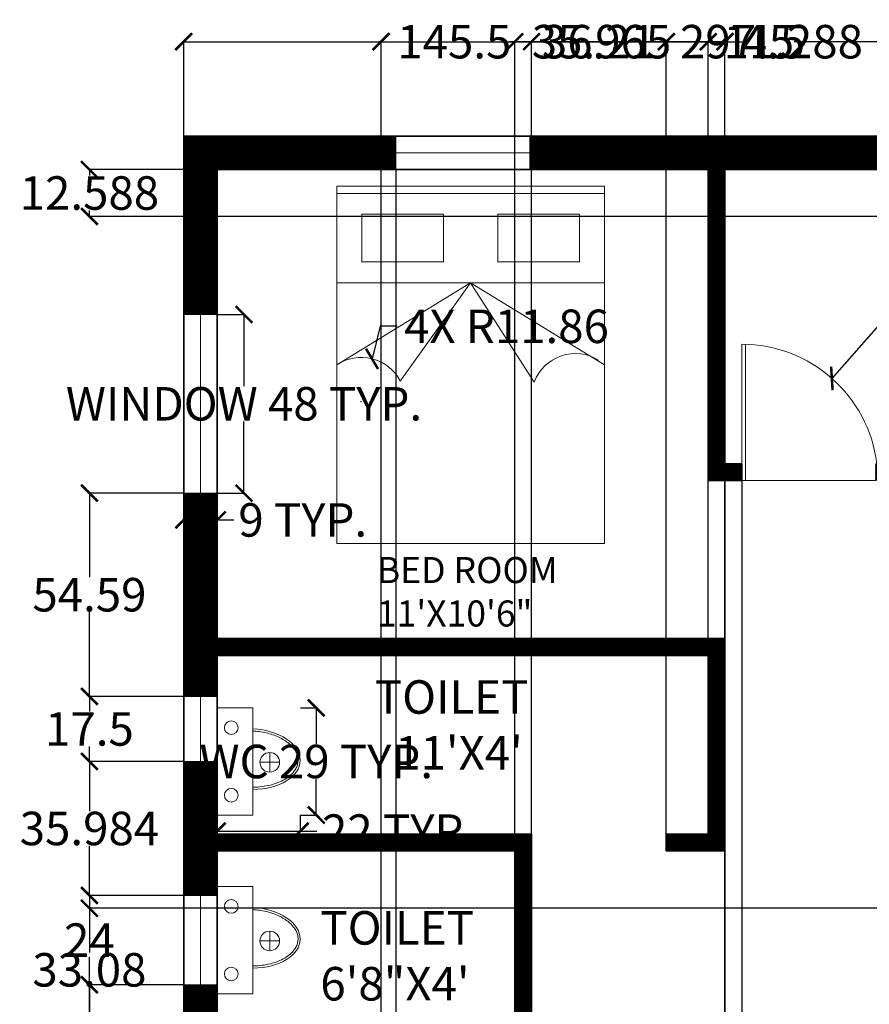
# Model space of a CAD drawing. Units: inches. Extents: x -1 to 426, y -6 to 532.
# Tile 3 of 4: x -1 to 228, y 267 to 532. Entities that reach past the tile are written whole.
import ezdxf

# ---------------------------------------------------------------- set-up
doc = ezdxf.new("R2010")
doc.units = ezdxf.units.IN
doc.header["$MEASUREMENT"] = 0
for name, color, linetype, lineweight in [('A-ANNO-DIMS', 2, 'Continuous', 18), ('A-AREA-IDEN', 7, 'Continuous', 25), ('A-DOOR', 3, 'Continuous', 18), ('A-FLOR-FIXT', 8, 'Continuous', 18), ('A-FURN', 8, 'Continuous', 18), ('A-GLAZ', 4, 'Continuous', 18)]:
    doc.layers.add(name, color=color, linetype=linetype, lineweight=lineweight)
doc.layers.add('A-WALL', color=159, linetype='Continuous', lineweight=35, true_color=0x223569)
doc.layers.add('A-WALL-PATT', color=177, linetype='Continuous', lineweight=13, true_color=0x2c4178)
doc.styles.get("Standard").update_dxf_attribs({"font": 'arial.ttf'})
doc.dimstyles.get("Standard").update_dxf_attribs({"dimtxt": 9, "dimasz": 4.5, "dimexe": 0.18, "dimexo": 0.0625, "dimgap": 0.09, "dimtad": 0, "dimtih": 1, "dimtoh": 1, "dimdec": 1, "dimzin": 0, "dimdsep": 46, "dimlunit": 4, "dimtxsty": 'Standard', "dimblk": 'ARCHTICK', "dimcen": 0.09, "dimadec": 0, "dimazin": 0, "dimtfac": 1, "dimtdec": 1, "dimtofl": 0, "dimtmove": 0, "dimatfit": 3, "dimfxl": 1, "dimtolj": 1, "dimtzin": 0, "dimarcsym": 0})

# ---------------------------------------------------------------- blocks, each defined once
blk = doc.blocks.new('WIN-36IN')
for p, q in [((0, 4.5), (36, 4.5)), ((0, -4.5), (0, 4.5)), ((36, 4.5), (36, -4.5)), ((0, 0), (36, 0)), ((36, -4.5), (0, -4.5))]:
    blk.add_line(p, q)
blk = doc.blocks.new('WIN-48IN')
for p, q in [((-4.5, 48), (4.5, 48)), ((-4.5, 0), (-4.5, 48)), ((0, 48), (0, 0)), ((4.5, 48), (4.5, 0)), ((4.5, 0), (-4.5, 0))]:
    blk.add_line(p, q)
blk = doc.blocks.new('BED-DOUBLE')
for p, q in [((-96, 0), (-96, 72)), ((-96, 72), (0, 72)), ((-26, 36), (-48, 72)), ((-26, 72), (-26, 0)), ((-2, 72), (-2, 0)), ((0, 72), (0, 0)), ((-52.33, 54.93), (-26, 36)), ((-26, 36), (-52.6, 18.9)), ((-48, 0), (-26, 36)), ((0, 0), (-96, 0))]:
    blk.add_line(p, q)
for points in [[(-7.5, 65.27), (-7.5, 43.28), (-20.33, 43.28), (-20.33, 65.27)], [(-7.5, 6.73), (-7.5, 28.72), (-20.33, 28.72), (-20.33, 6.73)]]:
    blk.add_lwpolyline(points, close=True)
for centre, start, end in [((-57.86, 65.42), 297.83, 33.7219), ((-56.81, 7.81), 328.371, 69.2037)]:
    blk.add_arc(centre, 11.86, start, end)
blk = doc.blocks.new('WC-TANK')
for p, q in [((0, -14.38), (0, 14.38)), ((0, 14.38), (9.6, 14.38)), ((9.6, 14.38), (9.6, 8.78)), ((9.6, -7.49), (9.6, 8.78)), ((14.13, -0.21), (14.13, 2.42)), ((14.13, 2.42), (14.13, -0.21)), ((14.13, -0.21), (11.49, -0.21)), ((11.49, -0.21), (14.13, -0.21)), ((14.13, -0.21), (16.76, -0.21)), ((16.76, -0.21), (14.13, -0.21)), ((14.13, -0.21), (14.13, -2.85)), ((9.6, -7.49), (9.6, -14.38)), ((9.6, -14.38), (0, -14.38))]:
    blk.add_line(p, q)
for centre, radius in [((3.77, 9.08), 1.84), ((14.13, -0.21), 2.63), ((3.77, -9.08), 1.84)]:
    blk.add_circle(centre, radius)
blk.add_ellipse((8.96, 0.66), major_axis=(13.35, -0.55), ratio=0.609473, start_param=4.785392, end_param=7.831087)
blk.add_open_spline([(9.6, -6.9), (10.03, -6.9), (10.47, -6.89), (11.69, -6.81), (12.46, -6.71), (13.95, -6.44), (14.67, -6.26), (16.04, -5.82), (16.69, -5.56), (17.88, -4.98), (18.43, -4.66), (19.41, -3.96), (19.84, -3.58), (20.51, -2.87), (20.76, -2.54), (21.18, -1.86), (21.35, -1.52), (21.59, -0.82), (21.67, -0.47), (21.74, 0.24), (21.73, 0.6), (21.63, 1.32), (21.53, 1.67), (21.25, 2.39), (21.07, 2.74), (20.61, 3.44), (20.33, 3.79), (19.7, 4.45), (19.34, 4.77), (18.55, 5.39), (18.12, 5.68), (17.18, 6.22), (16.67, 6.48), (15.61, 6.94), (15.05, 7.14), (13.89, 7.51), (13.29, 7.66), (12.06, 7.92), (11.43, 8.02), (10.38, 8.14), (9.98, 8.18), (9.57, 8.2)], degree=3, knots=[4.785392, 4.785392, 4.785392, 4.785392, 4.886226, 4.886226, 5.069344, 5.069344, 5.252462, 5.252462, 5.43558, 5.43558, 5.618699, 5.618699, 5.801817, 5.801817, 5.950651, 5.950651, 6.099486, 6.099486, 6.248321, 6.248321, 6.397155, 6.397155, 6.54599, 6.54599, 6.694824, 6.694824, 6.843659, 6.843659, 6.992494, 6.992494, 7.141328, 7.141328, 7.290163, 7.290163, 7.438998, 7.438998, 7.587832, 7.587832, 7.736667, 7.736667, 7.831087, 7.831087, 7.831087, 7.831087])
blk = doc.blocks.new('_ArchTick')
at = {"color": 0, "linetype": 'ByBlock', "const_width": 0.15}
blk.add_lwpolyline([(-0.5, -0.5), (0.5, 0.5)], dxfattribs=at)
blk = doc.blocks.new('*D9')
at = {"layer": 'A-ANNO-DIMS', "color": 0, "lineweight": -2, "transparency": 16777216}
for p, q in [((52.39, 452.57), (59.7, 452.57)), ((59.52, 452.57), (59.52, 433.32)), ((59.52, 404.57), (59.52, 423.82)), ((52.39, 404.57), (59.7, 404.57))]:
    blk.add_line(p, q, dxfattribs=at)
at = {"layer": 'Defpoints', "color": 0, "transparency": 16777216}
for p in [(52.32, 452.57), (59.52, 452.57), (52.32, 404.57)]:
    blk.add_point(p, dxfattribs=at)
at = {"layer": 'A-ANNO-DIMS', "color": 0, "lineweight": -2, "transparency": 16777216, "xscale": 4.5, "yscale": 4.5, "zscale": 4.5}
for p, rotation in [((59.52, 452.57), 90), ((59.52, 404.57), 270)]:
    blk.add_blockref('_ArchTick', p, dxfattribs=dict(at, rotation=rotation))
at = {"layer": 'A-ANNO-DIMS', "color": 0, "transparency": 16777216, "insert": (59.52, 428.57), "char_height": 9, "attachment_point": 5}
blk.add_mtext('\\A1;WINDOW 48 TYP.', dxfattribs=at)
blk = doc.blocks.new('*D10')
at = {"layer": 'A-ANNO-DIMS', "color": 0, "lineweight": -2, "transparency": 16777216}
for p, q in [((43.32, 404.51), (43.32, 397.19)), ((52.32, 404.51), (52.32, 397.19)), ((43.32, 397.37), (52.32, 397.37)), ((52.32, 397.37), (56.82, 397.37))]:
    blk.add_line(p, q, dxfattribs=at)
at = {"layer": 'Defpoints', "color": 0, "transparency": 16777216}
for p in [(43.32, 404.57), (52.32, 404.57), (52.32, 397.37)]:
    blk.add_point(p, dxfattribs=at)
at = {"layer": 'A-ANNO-DIMS', "color": 0, "lineweight": -2, "transparency": 16777216, "xscale": 4.5, "yscale": 4.5, "zscale": 4.5, "rotation": 180}
blk.add_blockref('_ArchTick', (43.32, 397.37), dxfattribs=at)
at = {"layer": 'A-ANNO-DIMS', "color": 0, "lineweight": -2, "transparency": 16777216, "xscale": 4.5, "yscale": 4.5, "zscale": 4.5}
blk.add_blockref('_ArchTick', (52.32, 397.37), dxfattribs=at)
at = {"layer": 'A-ANNO-DIMS', "color": 0, "transparency": 16777216, "insert": (75.32, 397.37), "char_height": 9, "attachment_point": 5}
blk.add_mtext('\\A1;9 TYP.', dxfattribs=at)
blk = doc.blocks.new('*D13')
at = {"layer": 'A-ANNO-DIMS', "color": 0, "lineweight": -2, "transparency": 16777216}
for p, q in [((74.7, 346.87), (79.13, 346.87)), ((78.95, 346.87), (78.95, 337.23)), ((78.95, 318.1), (78.95, 327.74)), ((74.7, 318.1), (79.13, 318.1))]:
    blk.add_line(p, q, dxfattribs=at)
at = {"layer": 'Defpoints', "color": 0, "transparency": 16777216}
for p in [(74.64, 346.87), (78.95, 346.87), (74.64, 318.1)]:
    blk.add_point(p, dxfattribs=at)
at = {"layer": 'A-ANNO-DIMS', "color": 0, "lineweight": -2, "transparency": 16777216, "xscale": 4.5, "yscale": 4.5, "zscale": 4.5}
for p, rotation in [((78.95, 346.87), 90), ((78.95, 318.1), 270)]:
    blk.add_blockref('_ArchTick', p, dxfattribs=dict(at, rotation=rotation))
at = {"layer": 'A-ANNO-DIMS', "color": 0, "transparency": 16777216, "insert": (78.95, 332.48), "char_height": 9, "attachment_point": 5}
blk.add_mtext('\\A1;WC 29 TYP.', dxfattribs=at)
blk = doc.blocks.new('*D14')
at = {"layer": 'A-ANNO-DIMS', "color": 0, "lineweight": -2, "transparency": 16777216}
for p, q in [((52.32, 318.03), (52.32, 313.6)), ((74.64, 318.03), (74.64, 313.6)), ((52.32, 313.78), (74.64, 313.78)), ((74.64, 313.78), (79.14, 313.78))]:
    blk.add_line(p, q, dxfattribs=at)
at = {"layer": 'Defpoints', "color": 0, "transparency": 16777216}
for p in [(52.32, 318.1), (74.64, 318.1), (74.64, 313.78)]:
    blk.add_point(p, dxfattribs=at)
at = {"layer": 'A-ANNO-DIMS', "color": 0, "lineweight": -2, "transparency": 16777216, "xscale": 4.5, "yscale": 4.5, "zscale": 4.5, "rotation": 180}
blk.add_blockref('_ArchTick', (52.32, 313.78), dxfattribs=at)
at = {"layer": 'A-ANNO-DIMS', "color": 0, "lineweight": -2, "transparency": 16777216, "xscale": 4.5, "yscale": 4.5, "zscale": 4.5}
blk.add_blockref('_ArchTick', (74.64, 313.78), dxfattribs=at)
at = {"layer": 'A-ANNO-DIMS', "color": 0, "transparency": 16777216, "insert": (101.21, 313.78), "char_height": 9, "attachment_point": 5}
blk.add_mtext('\\A1;22 TYP.', dxfattribs=at)
blk = doc.blocks.new('*D17')
at = {"layer": 'A-ANNO-DIMS', "color": 0, "lineweight": -2, "transparency": 16777216}
for p, q in [((43.32, 500.54), (43.32, 526.02)), ((43.32, 525.84), (176.69, 525.84)), ((340.82, 525.84), (207.46, 525.84)), ((340.82, 500.54), (340.82, 526.02))]:
    blk.add_line(p, q, dxfattribs=at)
at = {"layer": 'Defpoints', "color": 0, "transparency": 16777216}
for p in [(340.82, 525.84), (43.32, 500.48), (340.82, 500.48)]:
    blk.add_point(p, dxfattribs=at)
at = {"layer": 'A-ANNO-DIMS', "color": 0, "lineweight": -2, "transparency": 16777216, "xscale": 4.5, "yscale": 4.5, "zscale": 4.5, "rotation": 180}
blk.add_blockref('_ArchTick', (43.32, 525.84), dxfattribs=at)
at = {"layer": 'A-ANNO-DIMS', "color": 0, "lineweight": -2, "transparency": 16777216, "xscale": 4.5, "yscale": 4.5, "zscale": 4.5}
blk.add_blockref('_ArchTick', (340.82, 525.84), dxfattribs=at)
at = {"layer": 'A-ANNO-DIMS', "color": 0, "transparency": 16777216, "insert": (192.07, 525.84), "char_height": 9, "attachment_point": 5}
blk.add_mtext('\\A1;297.5', dxfattribs=at)
blk = doc.blocks.new('*D20')
at = {"layer": 'A-ANNO-DIMS', "color": 0, "lineweight": -2, "transparency": 16777216}
for p, q in [((43.32, 67.04), (43.32, 526.02)), ((43.32, 525.84), (101.19, 525.84)), ((188.82, 525.84), (130.96, 525.84)), ((188.82, 67.04), (188.82, 526.02))]:
    blk.add_line(p, q, dxfattribs=at)
at = {"layer": 'Defpoints', "color": 0, "transparency": 16777216}
for p in [(188.82, 525.84), (43.32, 66.98), (188.82, 66.98)]:
    blk.add_point(p, dxfattribs=at)
at = {"layer": 'A-ANNO-DIMS', "color": 0, "lineweight": -2, "transparency": 16777216, "xscale": 4.5, "yscale": 4.5, "zscale": 4.5, "rotation": 180}
blk.add_blockref('_ArchTick', (43.32, 525.84), dxfattribs=at)
at = {"layer": 'A-ANNO-DIMS', "color": 0, "lineweight": -2, "transparency": 16777216, "xscale": 4.5, "yscale": 4.5, "zscale": 4.5}
blk.add_blockref('_ArchTick', (188.82, 525.84), dxfattribs=at)
at = {"layer": 'A-ANNO-DIMS', "color": 0, "transparency": 16777216, "insert": (116.07, 525.84), "char_height": 9, "attachment_point": 5}
blk.add_mtext('\\A1;145.5', dxfattribs=at)
blk = doc.blocks.new('*D22')
at = {"layer": 'A-ANNO-DIMS', "color": 0, "lineweight": -2, "transparency": 16777216}
for p, q in [((52.32, 491.42), (52.32, 5.45)), ((100.32, 491.42), (100.32, 5.45)), ((52.32, 5.63), (69.6, 5.63)), ((100.32, 5.63), (83.05, 5.63))]:
    blk.add_line(p, q, dxfattribs=at)
at = {"layer": 'Defpoints', "color": 0, "transparency": 16777216}
for p in [(52.32, 491.48), (100.32, 491.48), (100.32, 5.63)]:
    blk.add_point(p, dxfattribs=at)
at = {"layer": 'A-ANNO-DIMS', "color": 0, "lineweight": -2, "transparency": 16777216, "xscale": 4.5, "yscale": 4.5, "zscale": 4.5, "rotation": 180}
blk.add_blockref('_ArchTick', (52.32, 5.63), dxfattribs=at)
at = {"layer": 'A-ANNO-DIMS', "color": 0, "lineweight": -2, "transparency": 16777216, "xscale": 4.5, "yscale": 4.5, "zscale": 4.5}
blk.add_blockref('_ArchTick', (100.32, 5.63), dxfattribs=at)
at = {"layer": 'A-ANNO-DIMS', "color": 0, "transparency": 16777216, "insert": (76.32, 5.63), "char_height": 9, "attachment_point": 5}
blk.add_mtext('\\A1;48', dxfattribs=at)
blk = doc.blocks.new('*D26')
at = {"layer": 'A-ANNO-DIMS', "color": 0, "lineweight": -2, "transparency": 16777216}
for p, q in [((43.26, 272.5), (17.79, 272.5)), ((17.97, 272.5), (17.97, 234.11)), ((17.97, 186.36), (17.97, 224.74)), ((43.26, 186.36), (17.79, 186.36))]:
    blk.add_line(p, q, dxfattribs=at)
at = {"layer": 'Defpoints', "color": 0, "transparency": 16777216}
for p in [(17.97, 272.5), (43.32, 272.5), (43.32, 186.36)]:
    blk.add_point(p, dxfattribs=at)
at = {"layer": 'A-ANNO-DIMS', "color": 0, "lineweight": -2, "transparency": 16777216, "xscale": 4.5, "yscale": 4.5, "zscale": 4.5}
for p, rotation in [((17.97, 272.5), 90), ((17.97, 186.36), 270)]:
    blk.add_blockref('_ArchTick', p, dxfattribs=dict(at, rotation=rotation))
at = {"layer": 'A-ANNO-DIMS', "color": 0, "transparency": 16777216, "insert": (17.97, 229.43), "char_height": 9, "attachment_point": 5}
blk.add_mtext('\\A1;86.14', dxfattribs=at)
blk = doc.blocks.new('*D27')
at = {"layer": 'A-ANNO-DIMS', "color": 0, "lineweight": -2, "transparency": 16777216}
for p, q in [((43.26, 296.5), (17.79, 296.5)), ((17.97, 296.5), (17.97, 289.11)), ((17.97, 272.5), (17.97, 279.89)), ((43.26, 272.5), (17.79, 272.5))]:
    blk.add_line(p, q, dxfattribs=at)
at = {"layer": 'Defpoints', "color": 0, "transparency": 16777216}
for p in [(17.97, 296.5), (43.32, 296.5), (43.32, 272.5)]:
    blk.add_point(p, dxfattribs=at)
at = {"layer": 'A-ANNO-DIMS', "color": 0, "lineweight": -2, "transparency": 16777216, "xscale": 4.5, "yscale": 4.5, "zscale": 4.5}
for p, rotation in [((17.97, 296.5), 90), ((17.97, 272.5), 270)]:
    blk.add_blockref('_ArchTick', p, dxfattribs=dict(at, rotation=rotation))
at = {"layer": 'A-ANNO-DIMS', "color": 0, "transparency": 16777216, "insert": (17.97, 284.5), "char_height": 9, "attachment_point": 5}
blk.add_mtext('\\A1;24', dxfattribs=at)
blk = doc.blocks.new('*D28')
at = {"layer": 'A-ANNO-DIMS', "color": 0, "lineweight": -2, "transparency": 16777216}
for p, q in [((43.26, 332.48), (17.79, 332.48)), ((17.97, 332.48), (17.97, 319.18)), ((17.97, 296.5), (17.97, 309.8)), ((43.26, 296.5), (17.79, 296.5))]:
    blk.add_line(p, q, dxfattribs=at)
at = {"layer": 'Defpoints', "color": 0, "transparency": 16777216}
for p in [(17.97, 332.48), (43.32, 332.48), (43.32, 296.5)]:
    blk.add_point(p, dxfattribs=at)
at = {"layer": 'A-ANNO-DIMS', "color": 0, "lineweight": -2, "transparency": 16777216, "xscale": 4.5, "yscale": 4.5, "zscale": 4.5}
for p, rotation in [((17.97, 332.48), 90), ((17.97, 296.5), 270)]:
    blk.add_blockref('_ArchTick', p, dxfattribs=dict(at, rotation=rotation))
at = {"layer": 'A-ANNO-DIMS', "color": 0, "transparency": 16777216, "insert": (17.97, 314.49), "char_height": 9, "attachment_point": 5}
blk.add_mtext('\\A1;35.984', dxfattribs=at)
blk = doc.blocks.new('*D29')
at = {"layer": 'A-ANNO-DIMS', "color": 0, "lineweight": -2, "transparency": 16777216}
for p, q in [((43.26, 349.98), (17.79, 349.98)), ((17.97, 349.98), (17.97, 345.92)), ((17.97, 332.48), (17.97, 336.55)), ((43.26, 332.48), (17.79, 332.48))]:
    blk.add_line(p, q, dxfattribs=at)
at = {"layer": 'Defpoints', "color": 0, "transparency": 16777216}
for p in [(17.97, 349.98), (43.32, 349.98), (43.32, 332.48)]:
    blk.add_point(p, dxfattribs=at)
at = {"layer": 'A-ANNO-DIMS', "color": 0, "lineweight": -2, "transparency": 16777216, "xscale": 4.5, "yscale": 4.5, "zscale": 4.5}
for p, rotation in [((17.97, 349.98), 90), ((17.97, 332.48), 270)]:
    blk.add_blockref('_ArchTick', p, dxfattribs=dict(at, rotation=rotation))
at = {"layer": 'A-ANNO-DIMS', "color": 0, "transparency": 16777216, "insert": (17.97, 341.23), "char_height": 9, "attachment_point": 5}
blk.add_mtext('\\A1;17.5', dxfattribs=at)
blk = doc.blocks.new('*D30')
at = {"layer": 'A-ANNO-DIMS', "color": 0, "lineweight": -2, "transparency": 16777216}
for p, q in [((43.26, 404.57), (17.79, 404.57)), ((17.97, 404.57), (17.97, 381.96)), ((17.97, 349.98), (17.97, 372.59)), ((43.26, 349.98), (17.79, 349.98))]:
    blk.add_line(p, q, dxfattribs=at)
at = {"layer": 'Defpoints', "color": 0, "transparency": 16777216}
for p in [(17.97, 404.57), (43.32, 404.57), (43.32, 349.98)]:
    blk.add_point(p, dxfattribs=at)
at = {"layer": 'A-ANNO-DIMS', "color": 0, "lineweight": -2, "transparency": 16777216, "xscale": 4.5, "yscale": 4.5, "zscale": 4.5}
for p, rotation in [((17.97, 404.57), 90), ((17.97, 349.98), 270)]:
    blk.add_blockref('_ArchTick', p, dxfattribs=dict(at, rotation=rotation))
at = {"layer": 'A-ANNO-DIMS', "color": 0, "transparency": 16777216, "insert": (17.97, 377.28), "char_height": 9, "attachment_point": 5}
blk.add_mtext('\\A1;54.59', dxfattribs=at)
blk = doc.blocks.new('*D32')
at = {"layer": 'A-ANNO-DIMS', "color": 0, "lineweight": -2, "transparency": 16777216}
for p, q in [((331.76, 293.06), (17.79, 293.06)), ((17.97, 293.06), (17.97, 281.21)), ((17.97, 259.98), (17.97, 271.83)), ((331.76, 259.98), (17.79, 259.98))]:
    blk.add_line(p, q, dxfattribs=at)
at = {"layer": 'Defpoints', "color": 0, "transparency": 16777216}
for p in [(17.97, 293.06), (331.82, 293.06), (331.82, 259.98)]:
    blk.add_point(p, dxfattribs=at)
at = {"layer": 'A-ANNO-DIMS', "color": 0, "lineweight": -2, "transparency": 16777216, "xscale": 4.5, "yscale": 4.5, "zscale": 4.5}
for p, rotation in [((17.97, 293.06), 90), ((17.97, 259.98), 270)]:
    blk.add_blockref('_ArchTick', p, dxfattribs=dict(at, rotation=rotation))
at = {"layer": 'A-ANNO-DIMS', "color": 0, "transparency": 16777216, "insert": (17.97, 276.52), "char_height": 9, "attachment_point": 5}
blk.add_mtext('\\A1;33.08', dxfattribs=at)
blk = doc.blocks.new('*D33')
at = {"layer": 'A-ANNO-DIMS', "color": 0, "lineweight": -2, "transparency": 16777216}
for p, q in [((331.76, 491.48), (17.79, 491.48)), ((17.97, 491.48), (17.97, 489.87)), ((331.76, 478.89), (17.79, 478.89)), ((17.97, 478.89), (17.97, 480.5))]:
    blk.add_line(p, q, dxfattribs=at)
at = {"layer": 'Defpoints', "color": 0, "transparency": 16777216}
for p in [(17.97, 491.48), (331.82, 491.48), (331.82, 478.89)]:
    blk.add_point(p, dxfattribs=at)
at = {"layer": 'A-ANNO-DIMS', "color": 0, "lineweight": -2, "transparency": 16777216, "xscale": 4.5, "yscale": 4.5, "zscale": 4.5}
for p, rotation in [((17.97, 491.48), 90), ((17.97, 478.89), 270)]:
    blk.add_blockref('_ArchTick', p, dxfattribs=dict(at, rotation=rotation))
at = {"layer": 'A-ANNO-DIMS', "color": 0, "transparency": 16777216, "insert": (17.97, 485.19), "char_height": 9, "attachment_point": 5}
blk.add_mtext('\\A1;12.588', dxfattribs=at)
blk = doc.blocks.new('*D39')
at = {"layer": 'A-ANNO-DIMS', "color": 0, "lineweight": -2, "transparency": 16777216}
for p, q in [((96.36, 256.04), (96.36, 526.02)), ((96.36, 525.84), (132.32, 525.84)), ((132.32, 256.04), (132.32, 526.02)), ((132.32, 525.84), (136.82, 525.84))]:
    blk.add_line(p, q, dxfattribs=at)
at = {"layer": 'Defpoints', "color": 0, "transparency": 16777216}
for p in [(132.32, 525.84), (96.36, 255.98), (132.32, 255.98)]:
    blk.add_point(p, dxfattribs=at)
at = {"layer": 'A-ANNO-DIMS', "color": 0, "lineweight": -2, "transparency": 16777216, "xscale": 4.5, "yscale": 4.5, "zscale": 4.5, "rotation": 180}
blk.add_blockref('_ArchTick', (96.36, 525.84), dxfattribs=at)
at = {"layer": 'A-ANNO-DIMS', "color": 0, "lineweight": -2, "transparency": 16777216, "xscale": 4.5, "yscale": 4.5, "zscale": 4.5}
blk.add_blockref('_ArchTick', (132.32, 525.84), dxfattribs=at)
at = {"layer": 'A-ANNO-DIMS', "color": 0, "transparency": 16777216, "insert": (155.63, 525.84), "char_height": 9, "attachment_point": 5}
blk.add_mtext('\\A1;35.965', dxfattribs=at)
blk = doc.blocks.new('*D40')
at = {"layer": 'A-ANNO-DIMS', "color": 0, "lineweight": -2, "transparency": 16777216}
for p, q in [((136.82, 313.04), (136.82, 526.02)), ((136.82, 525.84), (140.53, 525.84)), ((173.04, 525.84), (169.33, 525.84)), ((173.04, 313.04), (173.04, 526.02))]:
    blk.add_line(p, q, dxfattribs=at)
at = {"layer": 'Defpoints', "color": 0, "transparency": 16777216}
for p in [(173.04, 525.84), (136.82, 312.98), (173.04, 312.98)]:
    blk.add_point(p, dxfattribs=at)
at = {"layer": 'A-ANNO-DIMS', "color": 0, "lineweight": -2, "transparency": 16777216, "xscale": 4.5, "yscale": 4.5, "zscale": 4.5, "rotation": 180}
blk.add_blockref('_ArchTick', (136.82, 525.84), dxfattribs=at)
at = {"layer": 'A-ANNO-DIMS', "color": 0, "lineweight": -2, "transparency": 16777216, "xscale": 4.5, "yscale": 4.5, "zscale": 4.5}
blk.add_blockref('_ArchTick', (173.04, 525.84), dxfattribs=at)
at = {"layer": 'A-ANNO-DIMS', "color": 0, "transparency": 16777216, "insert": (154.93, 525.84), "char_height": 9, "attachment_point": 5}
blk.add_mtext('\\A1;36.21', dxfattribs=at)
blk = doc.blocks.new('*D41')
at = {"layer": 'A-ANNO-DIMS', "color": 0, "lineweight": -2, "transparency": 16777216}
for p, q in [((184.32, 361.04), (184.32, 526.02)), ((184.32, 525.84), (188.82, 525.84)), ((188.82, 365.54), (188.82, 526.02)), ((188.82, 525.84), (193.32, 525.84))]:
    blk.add_line(p, q, dxfattribs=at)
at = {"layer": 'Defpoints', "color": 0, "transparency": 16777216}
for p in [(188.82, 525.84), (188.82, 365.48), (184.32, 360.98)]:
    blk.add_point(p, dxfattribs=at)
at = {"layer": 'A-ANNO-DIMS', "color": 0, "lineweight": -2, "transparency": 16777216, "xscale": 4.5, "yscale": 4.5, "zscale": 4.5, "rotation": 180}
blk.add_blockref('_ArchTick', (184.32, 525.84), dxfattribs=at)
at = {"layer": 'A-ANNO-DIMS', "color": 0, "lineweight": -2, "transparency": 16777216, "xscale": 4.5, "yscale": 4.5, "zscale": 4.5}
blk.add_blockref('_ArchTick', (188.82, 525.84), dxfattribs=at)
at = {"layer": 'A-ANNO-DIMS', "color": 0, "transparency": 16777216, "insert": (201.82, 525.84), "char_height": 9, "attachment_point": 5}
blk.add_mtext('\\A1;4.5', dxfattribs=at)
blk = doc.blocks.new('*D47')
at = {"layer": 'A-ANNO-DIMS', "color": 0, "lineweight": -2, "transparency": 16777216}
for p, q in [((188.82, 412.42), (188.82, 5.45)), ((193.32, 412.42), (193.32, 5.45)), ((188.82, 5.63), (193.32, 5.63)), ((193.32, 5.63), (197.82, 5.63))]:
    blk.add_line(p, q, dxfattribs=at)
at = {"layer": 'Defpoints', "color": 0, "transparency": 16777216}
for p in [(188.82, 412.48), (193.32, 412.48), (193.32, 5.63)]:
    blk.add_point(p, dxfattribs=at)
at = {"layer": 'A-ANNO-DIMS', "color": 0, "lineweight": -2, "transparency": 16777216, "xscale": 4.5, "yscale": 4.5, "zscale": 4.5, "rotation": 180}
blk.add_blockref('_ArchTick', (188.82, 5.63), dxfattribs=at)
at = {"layer": 'A-ANNO-DIMS', "color": 0, "lineweight": -2, "transparency": 16777216, "xscale": 4.5, "yscale": 4.5, "zscale": 4.5}
blk.add_blockref('_ArchTick', (193.32, 5.63), dxfattribs=at)
at = {"layer": 'A-ANNO-DIMS', "color": 0, "transparency": 16777216, "insert": (206.32, 5.63), "char_height": 9, "attachment_point": 5}
blk.add_mtext('\\A1;4.5', dxfattribs=at)
blk = doc.blocks.new('*D50')
at = {"layer": 'A-ANNO-DIMS', "color": 0, "lineweight": -2, "transparency": 16777216}
for p, q in [((173.04, 313.04), (173.04, 526.02)), ((173.04, 525.84), (184.32, 525.84)), ((184.32, 313.04), (184.32, 526.02)), ((184.32, 525.84), (188.82, 525.84))]:
    blk.add_line(p, q, dxfattribs=at)
at = {"layer": 'Defpoints', "color": 0, "transparency": 16777216}
for p in [(184.32, 525.84), (173.04, 312.98), (184.32, 312.98)]:
    blk.add_point(p, dxfattribs=at)
at = {"layer": 'A-ANNO-DIMS', "color": 0, "lineweight": -2, "transparency": 16777216, "xscale": 4.5, "yscale": 4.5, "zscale": 4.5, "rotation": 180}
blk.add_blockref('_ArchTick', (173.04, 525.84), dxfattribs=at)
at = {"layer": 'A-ANNO-DIMS', "color": 0, "lineweight": -2, "transparency": 16777216, "xscale": 4.5, "yscale": 4.5, "zscale": 4.5}
blk.add_blockref('_ArchTick', (184.32, 525.84), dxfattribs=at)
at = {"layer": 'A-ANNO-DIMS', "color": 0, "transparency": 16777216, "insert": (207.18, 525.84), "char_height": 9, "attachment_point": 5}
blk.add_mtext('\\A1;11.288', dxfattribs=at)
blk = doc.blocks.new('*D55')
at = {"layer": 'A-ANNO-DIMS', "color": 0, "lineweight": -2, "transparency": 16777216}
for p, q in [((232.09, 451.85), (217.55, 435.4)), ((236.59, 451.85), (232.09, 451.85)), ((193.23, 407.98), (193.41, 407.98)), ((193.32, 407.89), (193.32, 408.07))]:
    blk.add_line(p, q, dxfattribs=at)
at = {"layer": 'Defpoints', "color": 0, "transparency": 16777216}
for p in [(217.55, 435.4), (193.32, 407.98)]:
    blk.add_point(p, dxfattribs=at)
at = {"layer": 'A-ANNO-DIMS', "color": 0, "lineweight": -2, "transparency": 16777216, "xscale": 4.5, "yscale": 4.5, "zscale": 4.5, "rotation": 228.5330341154112}
blk.add_blockref('_ArchTick', (217.55, 435.4), dxfattribs=at)
at = {"layer": 'A-ANNO-DIMS', "color": 0, "transparency": 16777216, "insert": (259.7, 451.85), "char_height": 9, "attachment_point": 5}
blk.add_mtext('\\A1;R36.585', dxfattribs=at)
blk = doc.blocks.new('*D57')
at = {"layer": 'A-ANNO-DIMS', "color": 0, "lineweight": -2, "transparency": 16777216}
for p, q in [((96.16, 449.38), (93.94, 440.65)), ((100.66, 449.38), (96.16, 449.38)), ((90.94, 429.15), (91.12, 429.15)), ((91.03, 429.06), (91.03, 429.24))]:
    blk.add_line(p, q, dxfattribs=at)
at = {"layer": 'Defpoints', "color": 0, "transparency": 16777216}
for p in [(93.94, 440.65), (91.03, 429.15)]:
    blk.add_point(p, dxfattribs=at)
at = {"layer": 'A-ANNO-DIMS', "color": 0, "lineweight": -2, "transparency": 16777216, "xscale": 4.5, "yscale": 4.5, "zscale": 4.5, "rotation": 255.7751302601228}
blk.add_blockref('_ArchTick', (93.94, 440.65), dxfattribs=at)
at = {"layer": 'A-ANNO-DIMS', "color": 0, "transparency": 16777216, "insert": (130.09, 449.38), "char_height": 9, "attachment_point": 5}
blk.add_mtext('\\A1;4X R11.86', dxfattribs=at)

msp = doc.modelspace()

# ---------------------------------------------------------------- hatches: boundary and pattern name
at = {"layer": 'A-WALL-PATT'}
h = msp.add_hatch(dxfattribs=at)
h.set_pattern_fill('ANSI31', color=256)
h.set_pattern_definition([(45, (-574.8435, 0), (-0.088388348, 0.088388348), [])])
h.paths.add_polyline_path([(100.3238, 500.4824), (43.3238, 500.4824), (43.3238, 452.5693), (52.3238, 452.5693), (52.3238, 491.4824), (100.3238, 491.4824)])
h.paths.add_polyline_path([(242.3238, 500.4824), (136.3238, 500.4824), (136.3238, 491.4824), (184.3238, 491.4824), (184.3238, 407.9824), (188.8238, 407.9824), (193.3238, 407.9824), (193.3238, 412.4824), (188.8238, 412.4824), (188.8238, 491.4824), (242.3238, 491.4824)])
h.paths.add_polyline_path([(340.8238, 500.4824), (278.3238, 500.4824), (278.3238, 491.4824), (331.8238, 491.4824), (331.8238, 478.8941), (340.8238, 478.8941)])
h.paths.add_polyline_path([(331.8238, 412.4824), (229.3238, 412.4824), (229.3238, 407.9824), (331.8238, 407.9824)])
h.paths.add_polyline_path([(340.8238, 430.8941), (331.8238, 430.8941), (331.8238, 341.0593), (340.8238, 341.0593)])
h.paths.add_polyline_path([(340.8238, 293.0593), (331.8238, 293.0593), (331.8238, 259.9824), (282.3238, 259.9824), (282.3238, 255.4824), (331.8238, 255.4824), (331.8238, 237.2917), (340.8238, 237.2917)])
h.paths.add_polyline_path([(340.8238, 153.5275), (340.8238, 201.2917), (331.8238, 201.2917), (331.8238, 177.4824), (241.8238, 177.4824), (241.8238, 255.4824), (246.3238, 255.4824), (246.3238, 259.9824), (237.3238, 259.9824), (237.3238, 255.4824), (237.3238, 172.9824), (331.8238, 172.9824), (331.8238, 153.5275), (331.8238, 75.9824), (237.3238, 75.9824), (237.3238, 66.9824), (340.8238, 66.9824)])
h.paths.add_polyline_path([(98.5766, 75.9824), (52.3238, 75.9824), (52.3238, 138.3606), (43.3238, 138.3606), (43.3238, 66.9824), (52.3238, 66.9824), (98.5766, 66.9824)])
h.paths.add_polyline_path([(188.8238, 75.9824), (188.8238, 153.5275), (188.8238, 209.4042, -0.02664097), (184.3238, 209.1642), (184.3238, 153.5275), (184.3238, 75.9824), (136.8238, 75.9824), (134.5766, 75.9824), (134.5766, 66.9824), (136.8238, 66.9824), (188.8238, 66.9824)])
h.paths.add_polyline_path([(52.3238, 255.9824), (96.3583, 255.9824), (96.3583, 260.4824), (52.3238, 260.4824), (52.3238, 272.4986), (43.3238, 272.4986), (43.3238, 186.3606), (52.3238, 186.3606)])
h.paths.add_polyline_path([(52.3238, 404.5693), (43.3238, 404.5693), (43.3238, 349.9808), (52.3238, 349.9808), (52.3238, 360.9824), (184.3238, 360.9824), (184.3238, 312.9824), (173.036, 312.9824), (173.036, 308.4824), (184.3238, 308.4824), (188.8238, 308.4824), (188.8238, 365.4824), (184.3238, 365.4824), (52.3238, 365.4824)])
h.paths.add_polyline_path([(188.8238, 260.4824), (136.8238, 260.4824), (136.8238, 308.4824), (136.8238, 312.9824), (52.3238, 312.9824), (52.3238, 332.4824), (43.3238, 332.4824), (43.3238, 308.4824), (43.3238, 296.4986), (52.3238, 296.4986), (52.3238, 298.8674), (52.3238, 308.4824), (132.3238, 308.4824), (132.3238, 260.4824), (132.3238, 255.9824), (136.8238, 255.9824), (184.3238, 255.9824), (184.3238, 251.4824), (186.5738, 251.4824), (188.8238, 251.4824), (188.8238, 255.9824)])

# ---------------------------------------------------------------- linework, layer by layer
at = {"layer": 'A-DOOR'}
for p, q in [((193.3238, 407.9824), (193.3238, 444.5678)), ((194.3238, 407.9824), (194.3238, 444.5541)), ((193.3238, 407.9824), (229.3238, 407.9824))]:
    msp.add_line(p, q, dxfattribs=at)
msp.add_arc((193.3238, 407.9824), 36.5854, 7.065274, 90, dxfattribs=at)
at = {"layer": 'A-GLAZ'}
for p, q in [((43.3238, 349.9808), (52.3238, 349.9808)), ((43.3238, 325.9808), (43.3238, 349.9808)), ((47.8238, 349.9808), (47.8238, 332.4824)), ((52.3238, 349.9808), (52.3238, 325.9808)), ((43.3238, 332.4824), (52.3238, 332.4824)), ((43.3238, 296.4986), (52.3238, 296.4986)), ((43.3238, 272.4986), (43.3238, 296.4986)), ((47.8238, 296.4986), (47.8238, 272.4986)), ((52.3238, 296.4986), (52.3238, 272.4986)), ((43.3238, 272.4986), (52.3238, 272.4986))]:
    msp.add_line(p, q, dxfattribs=at)
at = {"layer": 'A-WALL'}
for p, q in [((43.3238, 500.4824), (43.3238, 153.5275)), ((43.3238, 500.4824), (340.8238, 500.4824)), ((52.3238, 491.4824), (52.3238, 365.4824)), ((52.3238, 491.4824), (184.3238, 491.4824)), ((184.3238, 491.4824), (184.3238, 407.9824)), ((188.8238, 491.4824), (188.8238, 412.4824)), ((188.8238, 491.4824), (331.8238, 491.4824)), ((188.8238, 412.4824), (193.3238, 412.4824)), ((193.3238, 412.4824), (193.3238, 407.9824)), ((188.8238, 407.9824), (184.3238, 407.9824)), ((188.8238, 407.9824), (193.3238, 407.9824)), ((52.3238, 365.4824), (184.3238, 365.4824)), ((184.3238, 365.4824), (188.8238, 365.4824)), ((188.8238, 365.4824), (188.8238, 308.4824)), ((52.3238, 360.9824), (184.3238, 360.9824)), ((52.3238, 360.9824), (52.3238, 312.9824)), ((184.3238, 360.9824), (184.3238, 312.9824)), ((43.3238, 308.4824), (43.3238, 332.4824)), ((52.3238, 332.4824), (52.3238, 312.9824)), ((52.3238, 312.9824), (136.8238, 312.9824)), ((136.8238, 308.4824), (136.8238, 312.9824)), ((173.036, 312.9824), (173.036, 308.4824)), ((173.036, 312.9824), (184.3238, 312.9824)), ((52.3238, 308.4824), (132.3238, 308.4824)), ((52.3238, 308.4824), (52.3238, 260.4824)), ((132.3238, 308.4824), (132.3238, 260.4824)), ((136.8238, 308.4824), (136.8238, 260.4824)), ((173.036, 308.4824), (184.3238, 308.4824)), ((184.3238, 308.4824), (188.8238, 308.4824))]:
    msp.add_line(p, q, dxfattribs=at)

# ---------------------------------------------------------------- block references
at = {"layer": 'A-FLOR-FIXT'}
for p in [(52.3238, 332.4824), (52.3238, 284.4824)]:
    msp.add_blockref('WC-TANK', p, dxfattribs=at)
at = {"layer": 'A-FURN', "rotation": 90.00000000000007}
msp.add_blockref('BED-DOUBLE', (156.446, 487.0198), dxfattribs=at)
at = {"layer": 'A-GLAZ'}
for name, p in [('WIN-36IN', (100.3238, 495.9824)), ('WIN-48IN', (47.8238, 404.5693))]:
    msp.add_blockref(name, p, dxfattribs=at)

# ---------------------------------------------------------------- texts
at = {"layer": 'A-AREA-IDEN', "attachment_point": 1}
for s, insert, char_height in [('BED ROOM\\P11\'X10\'6"', (95.2507, 387.4041), 7), (" TOILET\\P   11'X4'", (91.9325, 354.3042), 9), ('TOILET\\P6\'8"X4\'', (80.0508, 292.2866), 9)]:
    msp.add_mtext_dynamic_manual_height_columns(s, width=229.541527, gutter_width=1, heights=[0], dxfattribs=dict(at, insert=insert, char_height=char_height))

# ---------------------------------------------------------------- dimensions: what is measured, and where the dimension line sits
at = {"layer": 'A-ANNO-DIMS'}
for base, p1, p2, override, picture, middle in [((340.8238, 525.8389), (43.3238, 500.4824), (340.8238, 500.4824), {"dimdec": 1, "dimlfac": 1, "dimrnd": 0, "dimzin": 0, "dimdsep": 46, "dimlunit": 2}, '*D17', (192.0738, 525.8389)), ((188.8238, 525.8389), (43.3238, 66.9824), (188.8238, 66.9824), {"dimdec": 1, "dimlfac": 1, "dimrnd": 0, "dimzin": 0, "dimdsep": 46, "dimlunit": 2}, '*D20', (116.0738, 525.8389)), ((132.32378, 525.83891), (96.35834, 255.98241), (132.32378, 255.98241), {"dimdec": 3, "dimlfac": 1, "dimrnd": 0, "dimzin": 0, "dimdsep": 46, "dimlunit": 2}, '*D39', (155.62592, 525.83891)), ((173.036, 525.8389), (136.8238, 312.9824), (173.036, 312.9824), {"dimdec": 2, "dimlfac": 1, "dimrnd": 0, "dimzin": 0, "dimdsep": 46, "dimlunit": 2}, '*D40', (154.9299, 525.8389)), ((184.3238, 525.8389), (173.036, 312.9824), (184.3238, 312.9824), {"dimdec": 3, "dimlfac": 1, "dimrnd": 0, "dimzin": 0, "dimdsep": 46, "dimlunit": 2}, '*D50', (207.1808, 525.8389)), ((188.8238, 525.8389), (184.3238, 360.9824), (188.8238, 365.4824), {"dimdec": 1, "dimlfac": 1, "dimrnd": 0, "dimzin": 0, "dimdsep": 46, "dimlunit": 2}, '*D41', (201.8214, 525.8389)), ((100.3238, 5.6259), (52.3238, 491.4824), (100.3238, 491.4824), {"dimdec": 0, "dimlfac": 1, "dimrnd": 0, "dimzin": 0, "dimdsep": 46, "dimlunit": 2}, '*D22', (76.3238, 5.6259)), ((193.3238, 5.6259), (188.8238, 412.4824), (193.3238, 412.4824), {"dimdec": 1, "dimlfac": 1, "dimrnd": 0, "dimzin": 0, "dimdsep": 46, "dimlunit": 2}, '*D47', (206.3214, 5.6259))]:
    dim = msp.add_linear_dim(base=base, p1=p1, p2=p2, dimstyle='Standard', override=override, dxfattribs=at)
    dim.commit()
    dim.dimension.update_dxf_attribs({"geometry": picture, "text_midpoint": middle})
for base, p1, p2, override, picture, middle in [((17.9673, 491.4824), (331.8238, 478.8941), (331.8238, 491.4824), {"dimdec": 3, "dimlfac": 1, "dimrnd": 0, "dimzin": 0, "dimdsep": 46, "dimlunit": 2}, '*D33', (17.9673, 485.1883)), ((17.9673, 404.5693), (43.3238, 349.9808), (43.3238, 404.5693), {"dimdec": 2, "dimlfac": 1, "dimrnd": 0, "dimzin": 0, "dimdsep": 46, "dimlunit": 2}, '*D30', (17.9673, 377.275)), ((17.9673, 349.9808), (43.3238, 332.4824), (43.3238, 349.9808), {"dimdec": 1, "dimlfac": 1, "dimrnd": 0, "dimzin": 0, "dimdsep": 46, "dimlunit": 2}, '*D29', (17.9673, 341.2316)), ((17.9673, 332.4824), (43.3238, 296.4986), (43.3238, 332.4824), {"dimdec": 3, "dimlfac": 1, "dimrnd": 0, "dimzin": 0, "dimdsep": 46, "dimlunit": 2}, '*D28', (17.9673, 314.4905)), ((17.9673, 296.4986), (43.3238, 272.4986), (43.3238, 296.4986), {"dimdec": 0, "dimlfac": 1, "dimrnd": 0, "dimzin": 0, "dimdsep": 46, "dimlunit": 2}, '*D27', (17.9673, 284.4986)), ((17.9673, 293.0593), (331.8238, 259.9824), (331.8238, 293.0593), {"dimdec": 2, "dimlfac": 1, "dimrnd": 0, "dimzin": 0, "dimdsep": 46, "dimlunit": 2}, '*D32', (17.9673, 276.5209)), ((17.9673, 272.4986), (43.3238, 186.3606), (43.3238, 272.4986), {"dimdec": 2, "dimlfac": 1, "dimrnd": 0, "dimzin": 0, "dimdsep": 46, "dimlunit": 2}, '*D26', (17.9673, 229.4296))]:
    dim = msp.add_linear_dim(base=base, p1=p1, p2=p2, angle=90, dimstyle='Standard', override=override, dxfattribs=at)
    dim.commit()
    dim.dimension.update_dxf_attribs({"geometry": picture, "text_midpoint": middle})
dim = msp.add_radius_dim(center=(91.0305, 429.1549), mpoint=(93.9449, 440.6517), text='4X <>', dimstyle='Standard', override={"dimdec": 2, "dimlfac": 1, "dimrnd": 0, "dimzin": 0, "dimdsep": 46, "dimlunit": 2}, dxfattribs=at)
dim.commit()
dim.dimension.update_dxf_attribs({"geometry": '*D57', "text_midpoint": (130.0855, 449.3758)})
dim = msp.add_radius_dim(center=(193.3238, 407.9824), mpoint=(217.5502, 435.3972), dimstyle='Standard', override={"dimdec": 3, "dimlfac": 1, "dimrnd": 0, "dimzin": 0, "dimdsep": 46, "dimlunit": 2}, dxfattribs=at)
dim.commit()
dim.dimension.update_dxf_attribs({"geometry": '*D55', "text_midpoint": (259.6978, 451.8461), "dimtype": 164})
for base, p1, p2, text, picture, middle in [((59.5238, 452.5693), (52.3238, 404.5693), (52.3238, 452.5693), 'WINDOW <> TYP.', '*D9', (59.5238, 428.5693)), ((78.9529, 346.8674), (74.6374, 318.0975), (74.6374, 346.8674), 'WC <> TYP.', '*D13', (78.9529, 332.4824))]:
    dim = msp.add_linear_dim(base=base, p1=p1, p2=p2, angle=90, text=text, dimstyle='Standard', override={"dimdec": 0, "dimlfac": 1, "dimrnd": 0, "dimzin": 0, "dimdsep": 46, "dimlunit": 2}, dxfattribs=at)
    dim.commit()
    dim.dimension.update_dxf_attribs({"geometry": picture, "text_midpoint": middle})
for base, p1, p2, picture, middle in [((52.3238, 397.3693), (43.3238, 404.5693), (52.3238, 404.5693), '*D10', (75.322, 397.3693)), ((74.6374, 313.782), (52.3238, 318.0975), (74.6374, 318.0975), '*D14', (101.2087, 313.782))]:
    dim = msp.add_linear_dim(base=base, p1=p1, p2=p2, text='<> TYP.', dimstyle='Standard', override={"dimdec": 0, "dimlfac": 1, "dimrnd": 0, "dimzin": 0, "dimdsep": 46, "dimlunit": 2}, dxfattribs=at)
    dim.commit()
    dim.dimension.update_dxf_attribs({"geometry": picture, "text_midpoint": middle})

doc.saveas('drawing.dxf')
